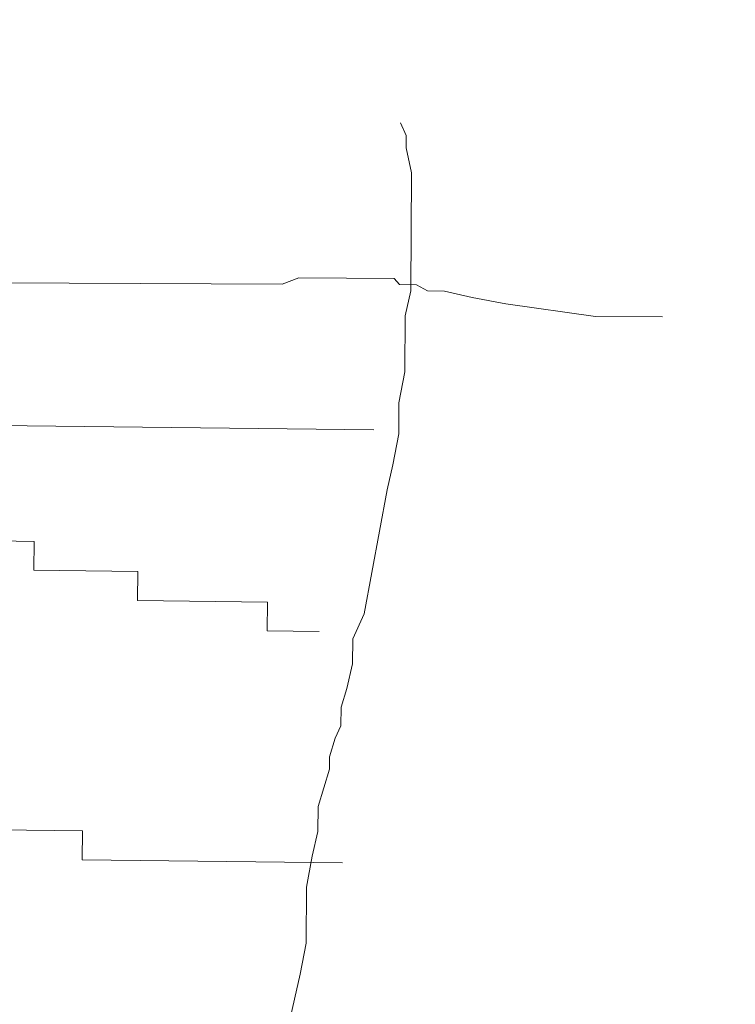
# Model space of a CAD drawing. Units: inches. Extents: x -466983 to 1020, y 324 to 318697.
# Tile 82 of 97: x 659.546 to 662.966, y 944.006 to 948.713. Entities that reach past the tile are written whole.
import ezdxf

# ---------------------------------------------------------------- set-up
doc = ezdxf.new("R2010")
doc.units = ezdxf.units.IN
doc.header["$MEASUREMENT"] = 0
doc.layers.add('A-FLOR-PATT', color=252, linetype='Continuous', lineweight=13)
doc.layers.add('A-FURN', color=8, linetype='Continuous', lineweight=18)

# ---------------------------------------------------------------- blocks, each defined once
blk = doc.blocks.new('L Shaped Sofa')
at = {"ltscale": 2}
for p, q in [((2387.5583, 741.0845), (2387.6585, 741.5177)), ((2387.5078, 740.8136), (2387.5583, 741.0845)), ((2387.5048, 740.3257), (2387.5078, 740.8136)), ((2387.4544, 740.0548), (2387.5048, 740.3257)), ((2387.1897, 740.1136), (2389.4581, 740.0859)), ((2387.4042, 739.8382), (2387.4544, 740.0548)), ((2389.4581, 740.0859), (2389.455, 739.834)), ((2387.4029, 739.6213), (2387.4042, 739.8382)), ((2389.455, 739.834), (2390.5892, 739.8201)), ((2387.3033, 739.2965), (2387.4029, 739.6213)), ((2387.3027, 739.1881), (2387.3033, 739.2965)), ((2387.2529, 739.0256), (2387.3027, 739.1881)), ((2387.2034, 738.9174), (2387.2529, 739.0256)), ((2387.2024, 738.7548), (2387.2034, 738.9174)), ((2387.1526, 738.5924), (2387.2024, 738.7548)), ((2387.1025, 738.3757), (2387.1526, 738.5924)), ((2387.1012, 738.1589), (2387.1025, 738.3757)), ((2387.0023, 737.9425), (2387.1012, 738.1589)), ((2387.3919, 738.0956), (2387.8456, 738.09)), ((2387.8456, 738.09), (2387.8425, 737.8381)), ((2386.8004, 736.8591), (2387.0023, 737.9425)), ((2387.8425, 737.8381), (2388.9767, 737.8242)), ((2388.9767, 737.8242), (2388.9736, 737.5723)), ((2388.9736, 737.5723), (2389.881, 737.5612)), ((2389.881, 737.5612), (2389.8779, 737.3093)), ((2389.8779, 737.3093), (2393.0536, 737.2705)), ((2386.7503, 736.6424), (2386.8004, 736.8591)), ((2386.6999, 736.3716), (2386.7503, 736.6424)), ((2386.6982, 736.1005), (2386.6999, 736.3716)), ((2386.9167, 736.3377), (2392.134, 736.274)), ((2386.6478, 735.8297), (2386.6982, 736.1005)), ((2386.6448, 735.3417), (2386.6478, 735.8297)), ((2384.4002, 735.3522), (2384.9857, 735.3495)), ((2384.9857, 735.3495), (2385.7658, 735.2374)), ((2386.5946, 735.1251), (2386.6448, 735.3417)), ((2385.7658, 735.2374), (2386.0582, 735.1818)), ((2386.0582, 735.1818), (2386.3019, 735.1264)), ((2386.3019, 735.1264), (2386.4483, 735.1258)), ((2386.4483, 735.1258), (2386.5455, 735.0711)), ((2386.5883, 734.095), (2386.5946, 735.1251)), ((2386.5455, 735.0711), (2386.6919, 735.0704)), ((2386.6919, 735.0704), (2386.7404, 735.016)), ((2387.5699, 735.0121), (2387.7166, 735.0656)), ((2387.7166, 735.0656), (2390.3515, 735.0532)), ((2386.7404, 735.016), (2387.5699, 735.0121)), ((2386.6358, 733.8779), (2386.5883, 734.095)), ((2386.6351, 733.7694), (2386.6358, 733.8779)), ((2386.6833, 733.6608), (2386.6351, 733.7694))]:
    blk.add_line(p, q, dxfattribs=at)

msp = doc.modelspace()

# ---------------------------------------------------------------- hatches: boundary and pattern name
at = {"layer": 'A-FLOR-PATT', "transparency": 33554572}
h = msp.add_hatch(dxfattribs=at)
h.set_pattern_fill('ANSI37', color=256, scale=30)
h.set_pattern_definition([(45, (-1212.4137, -290.035), (-2.6516504, 2.6516504), []), (135, (-1212.4137, -290.035), (-2.6516504, -2.6516504), [])])
h.paths.add_polyline_path([(901.8057, 1075.9377), (900.6144, 1075.9377), (900.6144, 1065.3856), (899.391, 1065.3856), (898.0911, 1065.3856), (892.8356, 1058.7098, -0.258377), (892.1875, 1058.3509), (879.9848, 1058.3509, -0.20177), (879.4382, 1058.5808), (874.0812, 1065.3856), (872.7813, 1065.3856), (871.5579, 1065.3856), (871.5579, 1075.9377), (813.8057, 1075.9377), (813.8057, 1044.7922), (832.3947, 1044.7922, -0.394795), (848.6602, 1028.5356), (848.6602, 1009.9377), (901.8057, 1009.9377), (901.8057, 1015.9377), (901.3057, 1015.9377), (871.3057, 1015.9377), (871.3057, 1017.2502), (871.3344, 1017.2502, -0.401453), (901.3057, 1045.9377), (901.8057, 1045.9377)])
edge = h.paths.add_edge_path(flags=16)
edge.add_line((847.7731, 1068.9486), (847.7731, 1073.7088))
edge.add_arc((849.2269, 1073.7088), 1.4538, 90, 180, ccw=False)
edge.add_line((849.2269, 1075.1627), (864.4921, 1075.1627))
edge.add_arc((864.4921, 1073.7088), 1.4538, 0, 90, ccw=False)
edge.add_line((865.9459, 1073.7088), (865.9459, 1069.0035))
edge.add_arc((832.6447, 1068.9761), 33.3012, -20.61234, 0.04725, ccw=False)
edge.add_ellipse((856.8595, 1058.48), major_axis=(0, 10.2131), ratio=0.6859192, start_angle=100.00884, end_angle=259.99116, ccw=False)
edge.add_arc((881.0742, 1068.9761), 33.3012, 180.04725, 200.61234, ccw=False)
h.paths.add_polyline_path([(853.1456, 1066.4815), (853.1456, 1066.4534), (853.1463, 1066.4534, 0.433107), (852.9166, 1066.6849), (852.9166, 1066.4534), (853.1456, 1066.4534), (853.1456, 1066.4815), (853.088, 1066.6122, 0.697939), (852.6995, 1066.4534), (852.7003, 1066.4534), (852.7003, 1066.4815), (852.9166, 1067.0012), (852.9166, 1066.6849, -0.396254)], flags=0)
h.paths.add_polyline_path([(861.0187, 1066.4815), (861.0187, 1066.4534), (861.0194, 1066.4534, 0.416404), (860.8024, 1066.6849), (860.8024, 1066.4534), (861.0187, 1066.4534), (861.0187, 1066.4815), (860.9672, 1066.6053, 0.713344), (860.5726, 1066.4534), (860.5734, 1066.4534), (860.5734, 1066.4815), (860.8024, 1067.0012), (860.8024, 1066.6849, -0.379973)], flags=0)
edge = h.paths.add_edge_path(flags=0)
edge.add_spline(control_points=[(861.1298, 1065.7855), (861.4661, 1065.2478), (861.6134, 1065.0161), (861.9833, 1064.3736), (862.1924, 1063.9443), (862.5614, 1063.0391), (862.7212, 1062.5633), (862.9865, 1061.5781), (863.092, 1061.0689), (863.2452, 1060.031), (863.293, 1059.5025), (863.3295, 1058.4409), (863.3181, 1057.9078), (863.2366, 1056.8518), (863.1664, 1056.3289), (862.9695, 1055.308), (862.8427, 1054.8099), (862.5365, 1053.8522), (862.3571, 1053.3927), (861.9514, 1052.5249), (861.7251, 1052.1166), (861.233, 1051.3622), (860.9672, 1051.0162), (860.4048, 1050.3949), (860.1082, 1050.1197), (859.4937, 1049.6461), (859.1758, 1049.4476), (858.5276, 1049.1299), (858.1973, 1049.0107), (857.5315, 1048.8518), (857.1959, 1048.8121), (856.5249, 1048.812), (856.1894, 1048.8515), (855.5236, 1049.0101), (855.1933, 1049.1291), (854.545, 1049.4465), (854.2271, 1049.6449), (853.6124, 1050.1183), (853.3158, 1050.3933), (852.7533, 1051.0143), (852.4874, 1051.3602), (851.9952, 1052.1144), (851.7688, 1052.5225), (851.3629, 1053.3902), (851.1834, 1053.8496), (850.877, 1054.8071), (850.7501, 1055.3051), (850.553, 1056.326), (850.4827, 1056.8488), (850.401, 1057.9048), (850.3895, 1058.4379), (850.4257, 1059.4995), (850.4734, 1060.0281), (850.6265, 1061.066), (850.7318, 1061.5753), (850.9969, 1062.5605), (851.1567, 1063.0365), (851.5254, 1063.9418), (851.7345, 1064.3712), (852.1056, 1065.0164), (852.2544, 1065.2503), (852.6082, 1065.7335)], knot_values=[3.915332, 3.915332, 3.915332, 3.915332, 4.013468, 4.013468, 4.175532, 4.175532, 4.337596, 4.337596, 4.49966, 4.49966, 4.661724, 4.661724, 4.823788, 4.823788, 4.985852, 4.985852, 5.147916, 5.147916, 5.30998, 5.30998, 5.472044, 5.472044, 5.634109, 5.634109, 5.796173, 5.796173, 5.958237, 5.958237, 6.120301, 6.120301, 6.282365, 6.282365, 6.444429, 6.444429, 6.606493, 6.606493, 6.768557, 6.768557, 6.930621, 6.930621, 7.092685, 7.092685, 7.254749, 7.254749, 7.416813, 7.416813, 7.578878, 7.578878, 7.740942, 7.740942, 7.903006, 7.903006, 8.06507, 8.06507, 8.227134, 8.227134, 8.389198, 8.389198, 8.551262, 8.551262, 8.65037, 8.65037, 8.65037, 8.65037], degree=3, periodic=0)
edge.add_line((852.6421, 1065.7855), (861.1298, 1065.7855))
edge = h.paths.add_edge_path(flags=0)
edge.add_ellipse((856.8496, 1057.7432), major_axis=(0, 7.7921), ratio=0.687861, start_angle=0, end_angle=360)
h.paths.add_polyline_path([(848.8634, 1069.3891), (848.8634, 1073.9605, -0.414214), (849.9538, 1075.0508), (863.7652, 1075.0508, -0.414214), (864.8555, 1073.9605), (864.8555, 1069.3891, -0.388936), (864.5237, 1069.027, -0.043561), (849.1953, 1069.027, -0.388936)], flags=0)
h.paths.add_polyline_path([(853.1006, 1068.1122, -1), (852.6775, 1068.1122, -1)], flags=0)
edge = h.paths.add_edge_path(flags=0)
edge.add_ellipse((856.8595, 1057.3378), major_axis=(0, 2.207), ratio=0.657164, start_angle=0, end_angle=360)
h.paths.add_polyline_path([(861.0415, 1068.1122, -1), (860.6184, 1068.1122, -1)], flags=0)
edge = h.paths.add_edge_path()
edge.add_line((573.9537, 1057.3412), (573.9537, 1075.9377))
edge.add_line((573.9537, 1075.9377), (558.7308, 1075.9377))
edge.add_line((558.7308, 1075.9377), (558.7308, 1065.3856))
edge.add_line((558.7308, 1065.3856), (557.5074, 1065.3856))
edge.add_line((557.5074, 1065.3856), (556.2075, 1065.3856))
edge.add_line((556.2075, 1065.3856), (550.952, 1058.7098))
edge.add_arc((550.3039, 1059.1155), 0.7646, 270, 327.9483, ccw=False)
edge.add_line((550.3039, 1058.3509), (538.1012, 1058.3509))
edge.add_arc((538.1012, 1059.1155), 0.7646, 224.3704, 270, ccw=False)
edge.add_line((537.5546, 1058.5808), (532.1976, 1065.3856))
edge.add_line((532.1976, 1065.3856), (530.8977, 1065.3856))
edge.add_line((530.8977, 1065.3856), (529.6743, 1065.3856))
edge.add_line((529.6743, 1065.3856), (529.6743, 1075.9377))
edge.add_line((529.6743, 1075.9377), (520.8057, 1075.9377))
edge.add_line((520.8057, 1075.9377), (520.8057, 1045.9377))
edge.add_line((520.8057, 1045.9377), (521.3057, 1045.9377))
edge.add_arc((521.3057, 1015.9377), 30, 2.50749, 90, ccw=False)
edge.add_line((551.277, 1017.2502), (551.3057, 1017.2502))
edge.add_line((551.3057, 1017.2502), (551.3057, 1015.9377))
edge.add_line((551.3057, 1015.9377), (520.8057, 1015.9377))
edge.add_line((520.8057, 1015.9377), (520.8057, 1009.9377))
edge.add_line((520.8057, 1009.9377), (559.1913, 1010.4022))
edge.add_arc((559.1913, 1011.856), 1.4538, 180, 270, ccw=False)
edge.add_line((557.7375, 1011.856), (557.7375, 1016.5613))
edge.add_arc((591.0386, 1016.5888), 33.3012, 159.38766, 180.04725, ccw=False)
edge.add_ellipse((566.8239, 1027.0848), major_axis=(0, 10.2131), ratio=0.6859192, start_angle=280.00884, end_angle=439.99116, ccw=False)
edge.add_arc((542.6091, 1016.5888), 33.3012, 0.04725, 20.61234, ccw=False)
edge.add_line((575.9103, 1016.6162), (575.9103, 1011.856))
edge.add_arc((574.4565, 1011.856), 1.4538, -90, 0, ccw=False)
edge.add_line((574.4565, 1010.4022), (608.8057, 1009.9377))
edge.add_line((608.8057, 1009.9377), (608.8057, 1041.0857))
edge.add_line((608.8057, 1041.0857), (590.2179, 1041.0857))
edge.add_arc((590.775, 1057.9074), 16.8309, 181.92775, 268.10321, ccw=False)
edge = h.paths.add_edge_path()
edge.add_ellipse((494.2443, 583.6204), major_axis=(0, 10.2131), ratio=0.6859192, start_angle=280.00884, end_angle=439.99116, ccw=False)
edge.add_arc((470.0296, 573.1243), 33.3012, 0.04725, 20.61234, ccw=False)
edge.add_line((503.3307, 573.1518), (503.3307, 568.3916))
edge.add_arc((501.8769, 568.3916), 1.4538, -90, 0, ccw=False)
edge.add_line((501.8769, 566.9377), (539.8057, 566.9377))
edge.add_line((539.8057, 566.9377), (539.8057, 572.9377))
edge.add_line((539.8057, 572.9377), (539.3057, 572.9377))
edge.add_line((539.3057, 572.9377), (509.3057, 572.9377))
edge.add_line((509.3057, 572.9377), (509.3057, 574.2502))
edge.add_line((509.3057, 574.2502), (509.3344, 574.2502))
edge.add_arc((539.3057, 572.9377), 30, 90, 177.49251, ccw=False)
edge.add_line((539.3057, 602.9377), (539.8057, 602.9377))
edge.add_line((539.8057, 602.9377), (539.8057, 626.9377))
edge.add_line((539.8057, 626.9377), (531.7718, 626.9377))
edge.add_line((531.7718, 626.9377), (531.7718, 616.3856))
edge.add_line((531.7718, 616.3856), (530.5484, 616.3856))
edge.add_line((530.5484, 616.3856), (529.2485, 616.3856))
edge.add_line((529.2485, 616.3856), (523.7105, 609.3509))
edge.add_line((523.7105, 609.3509), (510.7766, 609.3509))
edge.add_line((510.7766, 609.3509), (505.2386, 616.3856))
edge.add_line((505.2386, 616.3856), (503.9387, 616.3856))
edge.add_line((503.9387, 616.3856), (502.7153, 616.3856))
edge.add_line((502.7153, 616.3856), (502.7153, 626.9377))
edge.add_line((502.7153, 626.9377), (481.6983, 626.9377))
edge.add_line((481.6983, 626.9377), (481.6983, 610.995))
edge.add_arc((467.2703, 611.4728), 14.4359, 271.92775, 358.10321, ccw=False)
edge.add_line((467.7559, 597.0451), (451.8057, 597.0451))
edge.add_line((451.8057, 597.0451), (451.8057, 584.4035))
edge.add_line((451.8057, 584.4035), (451.8057, 566.9377))
edge.add_line((451.8057, 566.9377), (486.6117, 566.9377))
edge.add_arc((486.6117, 568.3916), 1.4538, 180, 270, ccw=False)
edge.add_line((485.1579, 568.3916), (485.1579, 573.0969))
edge.add_arc((518.4591, 573.1243), 33.3012, 159.38766, 180.04725, ccw=False)
h.paths.add_polyline_path([(836.2609, 1020.7328), (879.8898, 1020.7328), (879.8898, 1039.3902), (836.2609, 1039.3902)], flags=25)
h.paths.add_polyline_path([(549.9851, 1036.7492), (593.614, 1036.7492), (593.614, 1055.4065), (549.9851, 1055.4065)], flags=24)
h.paths.add_polyline_path([(475.123, 595.5959), (518.752, 595.5959), (518.752, 614.2532), (475.123, 614.2532)], flags=24)
h = msp.add_hatch(dxfattribs=at)
h.set_pattern_fill('ANSI37', color=256, scale=20)
h.set_pattern_definition([(45, (-1212.4137, -290.035), (-1.767767, 1.767767), []), (135, (-1212.4137, -290.035), (-1.767767, -1.767767), [])])
h.paths.add_polyline_path([(809.8057, 870.9377), (809.8057, 888.1519), (806.9985, 888.1519), (802.6624, 888.1519), (789.3832, 888.1519), (786.2846, 888.1519, -0.414214), (785.4991, 888.9374), (785.4991, 900.1959), (785.4991, 908.4696, -0.414214), (786.8082, 909.7787, -0.414214), (785.4991, 911.0878), (785.4991, 929.1015, -0.414214), (786.8082, 930.4106, -0.414214), (785.4991, 931.7197), (785.4991, 931.9039, -0.414214), (784.19, 930.5948), (766.7223, 930.5948, -0.412359), (765.4132, 931.8956, -0.413741), (764.1145, 930.5782), (744.5781, 930.422, -0.416556), (743.7864, 931.2075), (743.7864, 933.5153), (742.2154, 933.5153), (742.2154, 952.024, -0.001344), (743.7864, 952.1998), (743.7864, 953.9377), (678.5915, 953.9377), (678.5915, 951.1305), (678.5915, 946.7945), (678.5915, 933.5153), (678.5915, 930.4166, -0.414214), (677.806, 929.6312), (666.5475, 929.6312), (658.2738, 929.6312, -0.414214), (656.9647, 930.9403, -0.414214), (655.6556, 929.6312), (637.6419, 929.6312, -0.414214), (636.3328, 930.9403, -0.414214), (635.0237, 929.6312), (634.8395, 929.6312, -0.414214), (636.1486, 928.322), (636.1486, 910.8544, -0.412359), (634.8478, 909.5452, -0.413741), (636.1653, 908.2466), (636.3214, 888.7102, -0.416556), (635.5359, 887.9184), (633.2281, 887.9184), (633.2281, 886.3475), (614.7194, 886.3475, -0.001344), (614.5436, 887.9184), (612.8057, 887.9184), (612.8057, 834.9377), (612.8057, 752.9377), (612.8057, 748.9377), (612.8057, 697.9377), (654.8057, 697.9377), (654.8057, 701.9377), (715.8057, 701.9377), (715.8057, 737.4353), (774.2918, 737.4353), (774.2918, 795.9377), (809.8057, 795.9377)])
h.paths.add_polyline_path([(679.2761, 849.5757, 0.102523), (682.1475, 849.2608, -0.080461), (694.5428, 849.7725, -0.283899), (694.4822, 849.0082, 0.136605), (694.4068, 848.8103, -0.030441), (694.5428, 846.8929), (694.5428, 842.6198), (694.5428, 838.3466, -0.028219), (694.4246, 836.5684), (694.425, 836.5684, 0.196187), (694.4456, 836.2708, -0.302897), (694.5428, 835.467, -0.080461), (682.1475, 835.9787, 0.102523), (679.2761, 835.6638, -0.58611), (678.6457, 836.0169), (678.6457, 849.2227, -0.58611)], flags=16)
h.paths.add_polyline_path([(679.5173, 848.6515, 0.699597), (679.476, 848.6342, 1.20716), (679.1935, 848.7422, 0.010621)], flags=0)
h.paths.add_polyline_path([(679.4923, 836.5608, -0.013798), (679.9178, 836.6594, -0.071703), (682.8533, 837.1434, -0.165743), (682.1665, 839.1006), (682.1665, 842.6094), (682.1665, 846.0603, -0.240616), (683.4733, 848.6767, -0.068263), (693.9295, 849.0082), (693.7875, 848.7083), (693.7875, 849.0228, 0.067332), (683.4733, 848.6767, 0.240616), (682.1665, 846.0603), (682.1665, 842.6094), (682.1665, 839.1006, 0.23459), (683.461, 836.5513, 0.068093), (693.7875, 836.1955), (693.7875, 836.5104), (693.9296, 836.2102, -0.077215), (682.2421, 836.7815, 0.086627), (679.5283, 836.5701, -0.628402), (679.5029, 836.5735), (679.5029, 836.6071, 0.910458)], flags=0)
h.paths.add_polyline_path([(679.476, 848.6364), (679.2069, 848.647), (679.2069, 836.5718, 0.913566), (679.3645, 836.5861), (679.476, 836.5824)], flags=0)
h.paths.add_polyline_path([(679.2761, 829.8604, 0.102523), (682.1475, 829.5455, -0.080461), (694.5428, 830.0572, -0.283899), (694.4822, 829.2929, 0.136605), (694.4068, 829.095, -0.030441), (694.5428, 827.1776), (694.5428, 822.9045), (694.5428, 818.6314, -0.028219), (694.4246, 816.8531), (694.425, 816.8532, 0.196187), (694.4456, 816.5555, -0.302897), (694.5428, 815.7517, -0.080461), (682.1475, 816.2635, 0.102523), (679.2761, 815.9485, -0.58611), (678.6457, 816.3016), (678.6457, 829.5074, -0.58611)], flags=16)
h.paths.add_polyline_path([(679.5173, 828.9362, 0.699597), (679.476, 828.9189, 1.20716), (679.1935, 829.0269, 0.010621)], flags=0)
h.paths.add_polyline_path([(679.4923, 816.8456, -0.013798), (679.9178, 816.9441, -0.071703), (682.8533, 817.4281, -0.165743), (682.1665, 819.3853), (682.1665, 822.8941), (682.1665, 826.345, -0.240616), (683.4733, 828.9614, -0.068263), (693.9295, 829.2929), (693.7875, 828.9931), (693.7875, 829.3076, 0.067332), (683.4733, 828.9614, 0.240616), (682.1665, 826.345), (682.1665, 822.8941), (682.1665, 819.3853, 0.23459), (683.461, 816.836, 0.068093), (693.7875, 816.4802), (693.7875, 816.7952), (693.9296, 816.4949, -0.077215), (682.2421, 817.0662, 0.086627), (679.5283, 816.8549, -0.628402), (679.5029, 816.8582), (679.5029, 816.8918, 0.910458)], flags=0)
h.paths.add_polyline_path([(679.476, 828.9211), (679.2069, 828.9317), (679.2069, 816.8565, 0.913566), (679.3645, 816.8708), (679.476, 816.8671)], flags=0)
h.paths.add_polyline_path([(679.2761, 810.1451, 0.102523), (682.1475, 809.8302, -0.080461), (694.5428, 810.342, -0.3023), (694.4466, 809.5394, 0.10023), (694.4058, 809.3878, -0.03057), (694.5428, 807.4623), (694.5428, 803.1892), (694.5428, 798.9161, -0.03057), (694.4058, 796.9906, 0.10023), (694.4466, 796.839, -0.3023), (694.5428, 796.0365, -0.080461), (682.1475, 796.5482, 0.102523), (679.2761, 796.2333, -0.58611), (678.6457, 796.5863), (678.6457, 809.7921, -0.58611)], flags=16)
h.paths.add_polyline_path([(679.5173, 809.2417, 0.699597), (679.476, 809.2244, 1.20716), (679.1935, 809.3324, 0.010621)], flags=0)
h.paths.add_polyline_path([(679.4923, 797.151, -0.013798), (679.9178, 797.2496, -0.071703), (682.8533, 797.7336, -0.165743), (682.1665, 799.6908), (682.1665, 803.1996), (682.1665, 806.6505, -0.239349), (683.461, 809.2577, -0.072465), (694.4468, 809.5405, 0.197932), (694.425, 809.2405), (693.7875, 809.2985), (693.7875, 809.6135, 0.068093), (683.461, 809.2577, 0.239349), (682.1665, 806.6505), (682.1665, 803.1996), (682.1665, 799.6908, 0.235854), (683.4733, 797.1323, 0.067332), (693.7875, 796.7861), (693.7875, 797.1006), (694.425, 797.1586, 0.197932), (694.4468, 796.8586, -0.080419), (682.1557, 797.3795, 0.083867), (679.5283, 797.1603, -0.628402), (679.5029, 797.1637), (679.5029, 797.1973, 0.910458)], flags=0)
h.paths.add_polyline_path([(679.2069, 809.2372), (679.2069, 797.162, 0.913566), (679.3645, 797.1763), (679.476, 797.1726), (679.476, 809.2266)], flags=0)
h.paths.add_polyline_path([(695.3643, 853.2989), (728.2231, 853.2989), (728.2231, 771.1519), (695.3643, 771.1519)], flags=16)
h.paths.add_polyline_path([(696.0215, 852.6417), (727.5659, 852.6417), (727.5659, 771.809), (696.0215, 771.809)], flags=0)
h.paths.add_polyline_path([(679.2761, 788.7869, 0.102523), (682.1475, 788.472, -0.080461), (694.5428, 788.9837, -0.3023), (694.4466, 788.1812, 0.10023), (694.4058, 788.0296, -0.03057), (694.5428, 786.1041), (694.5428, 781.831), (694.5428, 777.5578, -0.03057), (694.4058, 775.6323, 0.10023), (694.4466, 775.4808, -0.3023), (694.5428, 774.6782, -0.080461), (682.1475, 775.19, 0.102523), (679.2761, 774.875, -0.58611), (678.6457, 775.2281), (678.6457, 788.4339, -0.58611)], flags=16)
h.paths.add_polyline_path([(679.5173, 787.8834, 0.699597), (679.476, 787.8662, 1.20716), (679.1935, 787.9742, 0.010621)], flags=0)
h.paths.add_polyline_path([(679.4923, 775.7928, -0.013798), (679.9178, 775.8914, -0.071703), (682.8533, 776.3753, -0.165743), (682.1665, 778.3325), (682.1665, 781.8414), (682.1665, 785.2922, -0.239349), (683.461, 787.8995, -0.072465), (694.4468, 788.1823, 0.197932), (694.425, 787.8823), (693.7875, 787.9403), (693.7875, 788.2553, 0.068093), (683.461, 787.8995, 0.239349), (682.1665, 785.2922), (682.1665, 781.8414), (682.1665, 778.3325, 0.235854), (683.4733, 775.7741, 0.067332), (693.7875, 775.4279), (693.7875, 775.7424), (694.425, 775.8004, 0.197932), (694.4468, 775.5004, -0.080419), (682.1557, 776.0212, 0.083867), (679.5283, 775.8021, -0.628402), (679.5029, 775.8054), (679.5029, 775.8391, 0.910458)], flags=0)
h.paths.add_polyline_path([(679.2069, 787.8789), (679.2069, 775.8038, 0.913566), (679.3645, 775.818), (679.476, 775.8144), (679.476, 787.8684)], flags=0)
h.paths.add_polyline_path([(704.641, 854.1204, -0.080461), (705.1527, 866.5157, 0.102523), (704.8378, 869.3871, -0.58611), (705.1908, 870.0174), (718.3966, 870.0174, -0.58611), (718.7496, 869.3871, 0.102523), (718.4347, 866.5157, -0.080461), (718.9465, 854.1204, -0.3023), (718.1439, 854.2166, 0.10023), (717.9924, 854.2574, -0.03057), (716.0668, 854.1204), (711.7937, 854.1204), (707.5206, 854.1204, -0.03057), (705.5951, 854.2574, 0.10023), (705.4435, 854.2166, -0.3023)], flags=16)
h.paths.add_polyline_path([(717.8462, 869.1459, 0.699597), (717.8289, 869.1872, 1.20716), (717.9369, 869.4697, 0.010621)], flags=0)
h.paths.add_polyline_path([(705.4631, 854.2164, -0.080419), (705.984, 866.5074, 0.083867), (705.7648, 869.1349, -0.628402), (705.7682, 869.1603), (705.8018, 869.1603, 0.910458), (705.7555, 869.1709, -0.013798), (705.8541, 868.7454, -0.071703), (706.3381, 865.8099, -0.165743), (708.2953, 866.4967), (711.8041, 866.4967), (715.255, 866.4967, -0.239349), (717.8622, 865.2022, -0.072465), (718.145, 854.2164, 0.197932), (717.845, 854.2382), (717.903, 854.8757), (718.218, 854.8757, 0.068093), (717.8622, 865.2022, 0.239349), (715.255, 866.4967), (711.8041, 866.4967), (708.2953, 866.4967, 0.235854), (705.7368, 865.1898, 0.067332), (705.3906, 854.8757), (705.7051, 854.8757), (705.7631, 854.2382, 0.197932)], flags=16)
h.paths.add_polyline_path([(705.7665, 869.4563, 0.913566), (705.7808, 869.2987), (705.7771, 869.1872), (717.8311, 869.1872), (717.8417, 869.4563)], flags=0)
h.paths.add_polyline_path([(729.0446, 842.6198), (729.0446, 846.8929, -0.03057), (729.1817, 848.8184, 0.10023), (729.1408, 848.9699, -0.3023), (729.0446, 849.7725, -0.080461), (741.4399, 849.2608, 0.102523), (744.3113, 849.5757, -0.58611), (744.9417, 849.2227), (744.9417, 836.0169, -0.58611), (744.3113, 835.6638, 0.102523), (741.4399, 835.9787, -0.080461), (729.0446, 835.467, -0.3023), (729.1408, 836.2696, 0.10023), (729.1817, 836.4211, -0.03057), (729.0446, 838.3466)], flags=16)
h.paths.add_polyline_path([(744.1115, 836.5846, 1.20716), (744.3939, 836.4766, 0.010621), (744.0701, 836.5673, 0.699597)], flags=0)
h.paths.add_polyline_path([(729.1407, 836.2684, 0.197932), (729.1624, 836.5684), (729.7999, 836.5104), (729.7999, 836.1955, 0.068093), (740.1264, 836.5513, 0.239349), (741.4209, 839.1585), (741.4209, 842.6094), (741.4209, 846.1182, 0.235854), (740.1141, 848.6767, 0.067332), (729.7999, 849.0228), (729.7999, 848.7083), (729.1624, 848.6503, 0.197932), (729.1407, 848.9504, -0.080419), (741.4317, 848.4295, 0.083867), (744.0591, 848.6486, -0.628402), (744.0845, 848.6453), (744.0845, 848.6117, 0.910458), (744.0951, 848.6579, -0.013798), (743.6696, 848.5594, -0.071703), (740.7341, 848.0754, -0.165743), (741.4209, 846.1182), (741.4209, 842.6094), (741.4209, 839.1585, -0.239349), (740.1264, 836.5513, -0.072465)], flags=0)
h.paths.add_polyline_path([(729.0446, 830.0572, -0.080461), (741.4399, 829.5455, 0.102523), (744.3113, 829.8604, -0.58611), (744.9417, 829.5074), (744.9417, 816.3016, -0.58611), (744.3113, 815.9485, 0.102523), (741.4399, 816.2635, -0.080461), (729.0446, 815.7517, -0.3023), (729.1408, 816.5543, 0.10023), (729.1817, 816.7058, -0.03057), (729.0446, 818.6314), (729.0446, 822.9045), (729.0446, 827.1776, -0.03057), (729.1817, 829.1031, 0.10023), (729.1408, 829.2547, -0.3023)], flags=16)
h.paths.add_polyline_path([(744.1115, 816.8693, 1.20716), (744.3939, 816.7613, 0.010621), (744.0701, 816.852, 0.699597)], flags=0)
h.paths.add_polyline_path([(729.1407, 829.2351, -0.080419), (741.4317, 828.7142, 0.083867), (744.0591, 828.9334, -0.628402), (744.0845, 828.93), (744.0845, 828.8964, 0.910458), (744.0951, 828.9427, -0.013798), (743.6696, 828.8441, -0.071703), (740.7341, 828.3601, -0.165743), (741.4209, 826.4029), (741.4209, 822.8941), (741.4209, 819.4432, -0.239349), (740.1264, 816.836, -0.072465), (729.1407, 816.5531, 0.197932), (729.1624, 816.8532), (729.7999, 816.7952), (729.7999, 816.4802, 0.068093), (740.1264, 816.836, 0.239349), (741.4209, 819.4432), (741.4209, 822.8941), (741.4209, 826.4029, 0.235854), (740.1141, 828.9614, 0.067332), (729.7999, 829.3076), (729.7999, 828.9931), (729.1624, 828.9351, 0.197932)], flags=16)
h.paths.add_polyline_path([(729.0446, 810.342, -0.080461), (741.4399, 809.8302, 0.102523), (744.3113, 810.1451, -0.58611), (744.9417, 809.7921), (744.9417, 796.5863, -0.58611), (744.3113, 796.2333, 0.102523), (741.4399, 796.5482, -0.080461), (729.0446, 796.0365, -0.283899), (729.1052, 796.8007, 0.136605), (729.1806, 796.9987, -0.030441), (729.0446, 798.9161), (729.0446, 803.1892), (729.0446, 807.4623, -0.028219), (729.1628, 809.2406), (729.1624, 809.2405, 0.196187), (729.1418, 809.5382, -0.302897)], flags=16)
h.paths.add_polyline_path([(744.1115, 797.1748, 1.20716), (744.3939, 797.0668, 0.010621), (744.0701, 797.1575, 0.699597)], flags=0)
h.paths.add_polyline_path([(741.3453, 809.0275, 0.086627), (744.0591, 809.2388, -0.628402), (744.0845, 809.2355), (744.0845, 809.2019, 0.910458), (744.0951, 809.2481, -0.013798), (743.6696, 809.1496, -0.071703), (740.7341, 808.6656, -0.165743), (741.4209, 806.7084), (741.4209, 803.1996), (741.4209, 799.7487, -0.240616), (740.1141, 797.1323, -0.068263), (729.658, 796.8008), (729.7999, 797.1006), (729.7999, 796.7861, 0.067332), (740.1141, 797.1323, 0.240616), (741.4209, 799.7487), (741.4209, 803.1996), (741.4209, 806.7084, 0.23459), (740.1264, 809.2577, 0.068093), (729.7999, 809.6135), (729.7999, 809.2985), (729.6578, 809.5988, -0.077215)], flags=0)
h.paths.add_polyline_path([(704.641, 770.3304, -0.283899), (705.4053, 770.2697, 0.136605), (705.6032, 770.1944, -0.030441), (707.5206, 770.3304), (711.7937, 770.3304), (716.0668, 770.3304, -0.028219), (717.8451, 770.2122), (717.845, 770.2126, 0.196187), (718.1427, 770.2331, -0.302897), (718.9465, 770.3304, -0.080461), (718.4347, 757.9351, 0.102523), (718.7496, 755.0637, -0.58611), (718.3966, 754.4333), (705.1908, 754.4333, -0.58611), (704.8378, 755.0637, 0.102523), (705.1527, 757.9351, -0.080461)], flags=16)
h.paths.add_polyline_path([(705.762, 755.3048, 0.699597), (705.7793, 755.2635, 1.20716), (705.6713, 754.9811, 0.010621)], flags=0)
h.paths.add_polyline_path([(705.4053, 769.717), (705.7051, 769.5751), (705.3906, 769.5751, 0.067332), (705.7368, 759.2609, 0.240616), (708.3532, 757.954), (711.8041, 757.954), (715.3129, 757.954, 0.23459), (717.8622, 759.2485, 0.068093), (718.218, 769.5751), (717.903, 769.5751), (718.2033, 769.7172, -0.077215), (717.632, 758.0297, 0.086627), (717.8433, 755.3159, -0.628402), (717.84, 755.2904), (717.8064, 755.2904, 0.910458), (717.8526, 755.2799, -0.013798), (717.7541, 755.7053, -0.071703), (717.2701, 758.6409, -0.165743), (715.3129, 757.954), (711.8041, 757.954), (708.3532, 757.954, -0.240616), (705.7368, 759.2609, -0.068263)], flags=0)
h.paths.add_polyline_path([(729.0446, 788.9837, -0.080461), (741.4399, 788.472, 0.102523), (744.3113, 788.7869, -0.58611), (744.9417, 788.4339), (744.9417, 775.2281, -0.58611), (744.3113, 774.875, 0.102523), (741.4399, 775.19, -0.080461), (729.0446, 774.6782, -0.283899), (729.1052, 775.4425, 0.136605), (729.1806, 775.6405, -0.030441), (729.0446, 777.5578), (729.0446, 781.831), (729.0446, 786.1041, -0.028219), (729.1628, 787.8823), (729.1624, 787.8823, 0.196187), (729.1418, 788.1799, -0.302897)], flags=16)
h.paths.add_polyline_path([(744.1115, 775.8165, 1.20716), (744.3939, 775.7086, 0.010621), (744.0701, 775.7993, 0.699597)], flags=0)
h.paths.add_polyline_path([(741.3453, 787.6692, 0.086627), (744.0591, 787.8806, -0.628402), (744.0845, 787.8773), (744.0845, 787.8437, 0.910458), (744.0951, 787.8899, -0.013798), (743.6696, 787.7913, -0.071703), (740.7341, 787.3074, -0.165743), (741.4209, 785.3502), (741.4209, 781.8414), (741.4209, 778.3905, -0.240616), (740.1141, 775.7741, -0.068263), (729.658, 775.4425), (729.7999, 775.7424), (729.7999, 775.4279, 0.067332), (740.1141, 775.7741, 0.240616), (741.4209, 778.3905), (741.4209, 781.8414), (741.4209, 785.3502, 0.23459), (740.1264, 787.8995, 0.068093), (729.7999, 788.2553), (729.7999, 787.9403), (729.6578, 788.2405, -0.077215)], flags=0)
h.paths.add_polyline_path([(744.1115, 848.6364), (744.1115, 836.5824), (744.3805, 836.5718), (744.3805, 848.647, 0.913566), (744.2229, 848.6327)], flags=0)
h.paths.add_polyline_path([(744.2229, 828.9174), (744.1115, 828.9211), (744.1115, 816.8671), (744.3805, 816.8565), (744.3805, 828.9317, 0.913566)], flags=0)
h.paths.add_polyline_path([(717.8311, 755.2635), (705.7771, 755.2635), (705.7665, 754.9945), (717.8417, 754.9945, 0.913566), (717.8274, 755.1521)], flags=0)
h.paths.add_polyline_path([(744.2229, 809.2229), (744.1115, 809.2266), (744.1115, 797.1726), (744.3805, 797.162), (744.3805, 809.2372, 0.913566)], flags=0)
h.paths.add_polyline_path([(744.1115, 787.8684), (744.1115, 775.8144), (744.3805, 775.8038), (744.3805, 787.8789, 0.913566), (744.2229, 787.8647)], flags=0)
h.paths.add_polyline_path([(678.8774, 877.1228), (737.6127, 877.1228), (737.6127, 899.5116), (678.8774, 899.5116)], flags=24)

# ---------------------------------------------------------------- linework, layer by layer
at = {"layer": 'A-FURN', "ltscale": 2}
for p, q in [((661.3663, 948.2191), (661.3927, 948.1595)), ((661.3663, 948.2191), (661.3927, 948.1595)), ((661.3663, 948.2191), (661.3927, 948.1595)), ((661.3663, 948.2191), (661.3927, 948.1595)), ((661.3663, 948.2191), (661.3927, 948.1595)), ((661.3663, 948.2191), (661.3927, 948.1595)), ((661.3927, 948.1595), (661.3924, 948.1001)), ((661.3927, 948.1595), (661.3924, 948.1001)), ((661.3927, 948.1595), (661.3924, 948.1001)), ((661.3927, 948.1595), (661.3924, 948.1001)), ((661.3927, 948.1595), (661.3924, 948.1001)), ((661.3927, 948.1595), (661.3924, 948.1001)), ((661.3924, 948.1001), (661.4184, 947.9811)), ((661.3924, 948.1001), (661.4184, 947.9811)), ((661.3924, 948.1001), (661.4184, 947.9811)), ((661.3924, 948.1001), (661.4184, 947.9811)), ((661.3924, 948.1001), (661.4184, 947.9811)), ((661.3924, 948.1001), (661.4184, 947.9811)), ((661.4184, 947.9811), (661.4149, 947.4163)), ((661.4184, 947.9811), (661.4149, 947.4163)), ((661.4184, 947.9811), (661.4149, 947.4163)), ((661.4184, 947.9811), (661.4149, 947.4163)), ((661.4184, 947.9811), (661.4149, 947.4163)), ((661.4184, 947.9811), (661.4149, 947.4163)), ((660.7999, 947.449), (659.3553, 947.4557)), ((660.7999, 947.449), (659.3553, 947.4557)), ((660.7999, 947.449), (659.3553, 947.4557)), ((660.7999, 947.449), (659.3553, 947.4557)), ((660.7999, 947.449), (659.3553, 947.4557)), ((660.7999, 947.449), (659.3553, 947.4557)), ((660.8803, 947.4783), (660.7999, 947.449)), ((660.8803, 947.4783), (660.7999, 947.449)), ((660.8803, 947.4783), (660.7999, 947.449)), ((660.8803, 947.4783), (660.7999, 947.449)), ((660.8803, 947.4783), (660.7999, 947.449)), ((660.8803, 947.4783), (660.7999, 947.449)), ((661.335, 947.4762), (660.8803, 947.4783)), ((661.335, 947.4762), (660.8803, 947.4783)), ((661.335, 947.4762), (660.8803, 947.4783)), ((661.335, 947.4762), (660.8803, 947.4783)), ((661.335, 947.4762), (660.8803, 947.4783)), ((661.335, 947.4762), (660.8803, 947.4783)), ((661.3616, 947.4463), (661.335, 947.4762)), ((661.3616, 947.4463), (661.335, 947.4762)), ((661.3616, 947.4463), (661.335, 947.4762)), ((661.3616, 947.4463), (661.335, 947.4762)), ((661.3616, 947.4463), (661.335, 947.4762)), ((661.3616, 947.4463), (661.335, 947.4762)), ((661.4419, 947.4459), (661.3616, 947.4463)), ((661.4419, 947.4459), (661.3616, 947.4463)), ((661.4419, 947.4459), (661.3616, 947.4463)), ((661.4419, 947.4459), (661.3616, 947.4463)), ((661.4419, 947.4459), (661.3616, 947.4463)), ((661.4419, 947.4459), (661.3616, 947.4463)), ((661.4952, 947.416), (661.4419, 947.4459)), ((661.4952, 947.416), (661.4419, 947.4459)), ((661.4952, 947.416), (661.4419, 947.4459)), ((661.4952, 947.416), (661.4419, 947.4459)), ((661.4952, 947.416), (661.4419, 947.4459)), ((661.4952, 947.416), (661.4419, 947.4459)), ((661.4149, 947.4163), (661.3874, 947.2976)), ((661.4149, 947.4163), (661.3874, 947.2976)), ((661.4149, 947.4163), (661.3874, 947.2976)), ((661.4149, 947.4163), (661.3874, 947.2976)), ((661.4149, 947.4163), (661.3874, 947.2976)), ((661.4149, 947.4163), (661.3874, 947.2976)), ((661.5754, 947.4156), (661.4952, 947.416)), ((661.5754, 947.4156), (661.4952, 947.416)), ((661.5754, 947.4156), (661.4952, 947.416)), ((661.5754, 947.4156), (661.4952, 947.416)), ((661.5754, 947.4156), (661.4952, 947.416)), ((661.5754, 947.4156), (661.4952, 947.416)), ((661.709, 947.3852), (661.5754, 947.4156)), ((661.709, 947.3852), (661.5754, 947.4156)), ((661.709, 947.3852), (661.5754, 947.4156)), ((661.709, 947.3852), (661.5754, 947.4156)), ((661.709, 947.3852), (661.5754, 947.4156)), ((661.709, 947.3852), (661.5754, 947.4156)), ((661.8693, 947.3548), (661.709, 947.3852)), ((661.8693, 947.3548), (661.709, 947.3852)), ((661.8693, 947.3548), (661.709, 947.3852)), ((661.8693, 947.3548), (661.709, 947.3852)), ((661.8693, 947.3548), (661.709, 947.3852)), ((661.8693, 947.3548), (661.709, 947.3852)), ((662.297, 947.2933), (661.8693, 947.3548)), ((662.297, 947.2933), (661.8693, 947.3548)), ((662.297, 947.2933), (661.8693, 947.3548)), ((662.297, 947.2933), (661.8693, 947.3548)), ((662.297, 947.2933), (661.8693, 947.3548)), ((662.297, 947.2933), (661.8693, 947.3548)), ((661.3874, 947.2976), (661.3858, 947.0301)), ((661.3874, 947.2976), (661.3858, 947.0301)), ((661.3874, 947.2976), (661.3858, 947.0301)), ((661.3874, 947.2976), (661.3858, 947.0301)), ((661.3874, 947.2976), (661.3858, 947.0301)), ((661.3874, 947.2976), (661.3858, 947.0301)), ((662.618, 947.2918), (662.297, 947.2933)), ((662.618, 947.2918), (662.297, 947.2933)), ((662.618, 947.2918), (662.297, 947.2933)), ((662.618, 947.2918), (662.297, 947.2933)), ((662.618, 947.2918), (662.297, 947.2933)), ((662.618, 947.2918), (662.297, 947.2933)), ((661.3858, 947.0301), (661.3582, 946.8816)), ((661.3858, 947.0301), (661.3582, 946.8816)), ((661.3858, 947.0301), (661.3582, 946.8816)), ((661.3858, 947.0301), (661.3582, 946.8816)), ((661.3858, 947.0301), (661.3582, 946.8816)), ((661.3858, 947.0301), (661.3582, 946.8816)), ((661.3582, 946.8816), (661.3572, 946.733)), ((661.3582, 946.8816), (661.3572, 946.733)), ((661.3582, 946.8816), (661.3572, 946.733)), ((661.3582, 946.8816), (661.3572, 946.733)), ((661.3582, 946.8816), (661.3572, 946.733)), ((661.3582, 946.8816), (661.3572, 946.733)), ((661.2384, 946.7516), (658.3782, 946.7865)), ((661.2384, 946.7516), (658.3782, 946.7865)), ((661.2384, 946.7516), (658.3782, 946.7865)), ((661.2384, 946.7516), (658.3782, 946.7865)), ((661.2384, 946.7516), (658.3782, 946.7865)), ((661.2384, 946.7516), (658.3782, 946.7865)), ((661.3572, 946.733), (661.3296, 946.5845)), ((661.3572, 946.733), (661.3296, 946.5845)), ((661.3572, 946.733), (661.3296, 946.5845)), ((661.3572, 946.733), (661.3296, 946.5845)), ((661.3572, 946.733), (661.3296, 946.5845)), ((661.3572, 946.733), (661.3296, 946.5845)), ((661.3296, 946.5845), (661.3021, 946.4657)), ((661.3296, 946.5845), (661.3021, 946.4657)), ((661.3296, 946.5845), (661.3021, 946.4657)), ((661.3296, 946.5845), (661.3021, 946.4657)), ((661.3296, 946.5845), (661.3021, 946.4657)), ((661.3296, 946.5845), (661.3021, 946.4657)), ((661.3021, 946.4657), (661.1915, 945.8718)), ((661.3021, 946.4657), (661.1915, 945.8718)), ((661.3021, 946.4657), (661.1915, 945.8718)), ((661.3021, 946.4657), (661.1915, 945.8718)), ((661.3021, 946.4657), (661.1915, 945.8718)), ((661.3021, 946.4657), (661.1915, 945.8718)), ((659.615, 946.2189), (657.874, 946.2402)), ((659.615, 946.2189), (657.874, 946.2402)), ((659.615, 946.2189), (657.874, 946.2402)), ((659.615, 946.2189), (657.874, 946.2402)), ((659.615, 946.2189), (657.874, 946.2402)), ((659.615, 946.2189), (657.874, 946.2402)), ((659.6133, 946.0808), (659.615, 946.2189)), ((659.6133, 946.0808), (659.615, 946.2189)), ((659.6133, 946.0808), (659.615, 946.2189)), ((659.6133, 946.0808), (659.615, 946.2189)), ((659.6133, 946.0808), (659.615, 946.2189)), ((659.6133, 946.0808), (659.615, 946.2189)), ((660.1107, 946.0747), (659.6133, 946.0808)), ((660.1107, 946.0747), (659.6133, 946.0808)), ((660.1107, 946.0747), (659.6133, 946.0808)), ((660.1107, 946.0747), (659.6133, 946.0808)), ((660.1107, 946.0747), (659.6133, 946.0808)), ((660.1107, 946.0747), (659.6133, 946.0808)), ((660.109, 945.9366), (660.1107, 946.0747)), ((660.109, 945.9366), (660.1107, 946.0747)), ((660.109, 945.9366), (660.1107, 946.0747)), ((660.109, 945.9366), (660.1107, 946.0747)), ((660.109, 945.9366), (660.1107, 946.0747)), ((660.109, 945.9366), (660.1107, 946.0747)), ((660.7308, 945.929), (660.109, 945.9366)), ((660.7308, 945.929), (660.109, 945.9366)), ((660.7308, 945.929), (660.109, 945.9366)), ((660.7308, 945.929), (660.109, 945.9366)), ((660.7308, 945.929), (660.109, 945.9366)), ((660.7308, 945.929), (660.109, 945.9366)), ((660.7291, 945.7909), (660.7308, 945.929)), ((660.7291, 945.7909), (660.7308, 945.929)), ((660.7291, 945.7909), (660.7308, 945.929)), ((660.7291, 945.7909), (660.7308, 945.929)), ((660.7291, 945.7909), (660.7308, 945.929)), ((660.7291, 945.7909), (660.7308, 945.929)), ((661.1915, 945.8718), (661.1372, 945.7532)), ((661.1915, 945.8718), (661.1372, 945.7532)), ((661.1915, 945.8718), (661.1372, 945.7532)), ((661.1915, 945.8718), (661.1372, 945.7532)), ((661.1915, 945.8718), (661.1372, 945.7532)), ((661.1915, 945.8718), (661.1372, 945.7532)), ((660.9778, 945.7879), (660.7291, 945.7909)), ((660.9778, 945.7879), (660.7291, 945.7909)), ((660.9778, 945.7879), (660.7291, 945.7909)), ((660.9778, 945.7879), (660.7291, 945.7909)), ((660.9778, 945.7879), (660.7291, 945.7909)), ((660.9778, 945.7879), (660.7291, 945.7909)), ((661.1372, 945.7532), (661.1365, 945.6343)), ((661.1372, 945.7532), (661.1365, 945.6343)), ((661.1372, 945.7532), (661.1365, 945.6343)), ((661.1372, 945.7532), (661.1365, 945.6343)), ((661.1372, 945.7532), (661.1365, 945.6343)), ((661.1372, 945.7532), (661.1365, 945.6343)), ((661.1365, 945.6343), (661.109, 945.5155)), ((661.1365, 945.6343), (661.109, 945.5155)), ((661.1365, 945.6343), (661.109, 945.5155)), ((661.1365, 945.6343), (661.109, 945.5155)), ((661.1365, 945.6343), (661.109, 945.5155)), ((661.1365, 945.6343), (661.109, 945.5155)), ((661.109, 945.5155), (661.0817, 945.4265)), ((661.109, 945.5155), (661.0817, 945.4265)), ((661.109, 945.5155), (661.0817, 945.4265)), ((661.109, 945.5155), (661.0817, 945.4265)), ((661.109, 945.5155), (661.0817, 945.4265)), ((661.109, 945.5155), (661.0817, 945.4265)), ((661.0817, 945.4265), (661.0812, 945.3373)), ((661.0817, 945.4265), (661.0812, 945.3373)), ((661.0817, 945.4265), (661.0812, 945.3373)), ((661.0817, 945.4265), (661.0812, 945.3373)), ((661.0817, 945.4265), (661.0812, 945.3373)), ((661.0817, 945.4265), (661.0812, 945.3373)), ((661.0812, 945.3373), (661.0541, 945.278)), ((661.0812, 945.3373), (661.0541, 945.278)), ((661.0812, 945.3373), (661.0541, 945.278)), ((661.0812, 945.3373), (661.0541, 945.278)), ((661.0812, 945.3373), (661.0541, 945.278)), ((661.0812, 945.3373), (661.0541, 945.278)), ((661.0541, 945.278), (661.0268, 945.189)), ((661.0541, 945.278), (661.0268, 945.189)), ((661.0541, 945.278), (661.0268, 945.189)), ((661.0541, 945.278), (661.0268, 945.189)), ((661.0541, 945.278), (661.0268, 945.189)), ((661.0541, 945.278), (661.0268, 945.189)), ((661.0268, 945.189), (661.0264, 945.1295)), ((661.0268, 945.189), (661.0264, 945.1295)), ((661.0268, 945.189), (661.0264, 945.1295)), ((661.0268, 945.189), (661.0264, 945.1295)), ((661.0268, 945.189), (661.0264, 945.1295)), ((661.0268, 945.189), (661.0264, 945.1295)), ((661.0264, 945.1295), (660.9718, 944.9514)), ((661.0264, 945.1295), (660.9718, 944.9514)), ((661.0264, 945.1295), (660.9718, 944.9514)), ((661.0264, 945.1295), (660.9718, 944.9514)), ((661.0264, 945.1295), (660.9718, 944.9514)), ((661.0264, 945.1295), (660.9718, 944.9514)), ((660.9718, 944.9514), (660.9711, 944.8325)), ((660.9718, 944.9514), (660.9711, 944.8325)), ((660.9718, 944.9514), (660.9711, 944.8325)), ((660.9718, 944.9514), (660.9711, 944.8325)), ((660.9718, 944.9514), (660.9711, 944.8325)), ((660.9718, 944.9514), (660.9711, 944.8325)), ((659.8468, 944.8348), (659.2251, 944.8424)), ((659.8468, 944.8348), (659.2251, 944.8424)), ((659.8468, 944.8348), (659.2251, 944.8424)), ((659.8468, 944.8348), (659.2251, 944.8424)), ((659.8468, 944.8348), (659.2251, 944.8424)), ((659.8468, 944.8348), (659.2251, 944.8424)), ((659.8451, 944.6967), (659.8468, 944.8348)), ((659.8451, 944.6967), (659.8468, 944.8348)), ((659.8451, 944.6967), (659.8468, 944.8348)), ((659.8451, 944.6967), (659.8468, 944.8348)), ((659.8451, 944.6967), (659.8468, 944.8348)), ((659.8451, 944.6967), (659.8468, 944.8348)), ((660.9711, 944.8325), (660.9436, 944.7138)), ((660.9711, 944.8325), (660.9436, 944.7138)), ((660.9711, 944.8325), (660.9436, 944.7138)), ((660.9711, 944.8325), (660.9436, 944.7138)), ((660.9711, 944.8325), (660.9436, 944.7138)), ((660.9711, 944.8325), (660.9436, 944.7138)), ((660.9436, 944.7138), (660.916, 944.5653)), ((660.9436, 944.7138), (660.916, 944.5653)), ((660.9436, 944.7138), (660.916, 944.5653)), ((660.9436, 944.7138), (660.916, 944.5653)), ((660.9436, 944.7138), (660.916, 944.5653)), ((660.9436, 944.7138), (660.916, 944.5653)), ((661.0887, 944.6815), (659.8451, 944.6967)), ((661.0887, 944.6815), (659.8451, 944.6967)), ((661.0887, 944.6815), (659.8451, 944.6967)), ((661.0887, 944.6815), (659.8451, 944.6967)), ((661.0887, 944.6815), (659.8451, 944.6967)), ((661.0887, 944.6815), (659.8451, 944.6967)), ((660.916, 944.5653), (660.9143, 944.2978)), ((660.916, 944.5653), (660.9143, 944.2978)), ((660.916, 944.5653), (660.9143, 944.2978)), ((660.916, 944.5653), (660.9143, 944.2978)), ((660.916, 944.5653), (660.9143, 944.2978)), ((660.916, 944.5653), (660.9143, 944.2978)), ((660.9143, 944.2978), (660.8867, 944.1493)), ((660.9143, 944.2978), (660.8867, 944.1493)), ((660.9143, 944.2978), (660.8867, 944.1493)), ((660.9143, 944.2978), (660.8867, 944.1493)), ((660.9143, 944.2978), (660.8867, 944.1493)), ((660.9143, 944.2978), (660.8867, 944.1493)), ((660.8867, 944.1493), (660.8317, 943.9118)), ((660.8867, 944.1493), (660.8317, 943.9118)), ((660.8867, 944.1493), (660.8317, 943.9118)), ((660.8867, 944.1493), (660.8317, 943.9118)), ((660.8867, 944.1493), (660.8317, 943.9118)), ((660.8867, 944.1493), (660.8317, 943.9118))]:
    msp.add_line(p, q, dxfattribs=at)

# ---------------------------------------------------------------- block references
at = {"layer": 'A-FURN', "xscale": 0.5482153745360612, "yscale": 0.5482153745360612, "zscale": 0.5482153745360612, "rotation": 180}
msp.add_blockref('L Shaped Sofa', (1969.7828, 1350.4232), dxfattribs=at)

doc.saveas('drawing.dxf')
